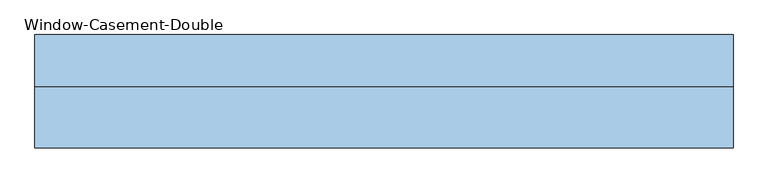
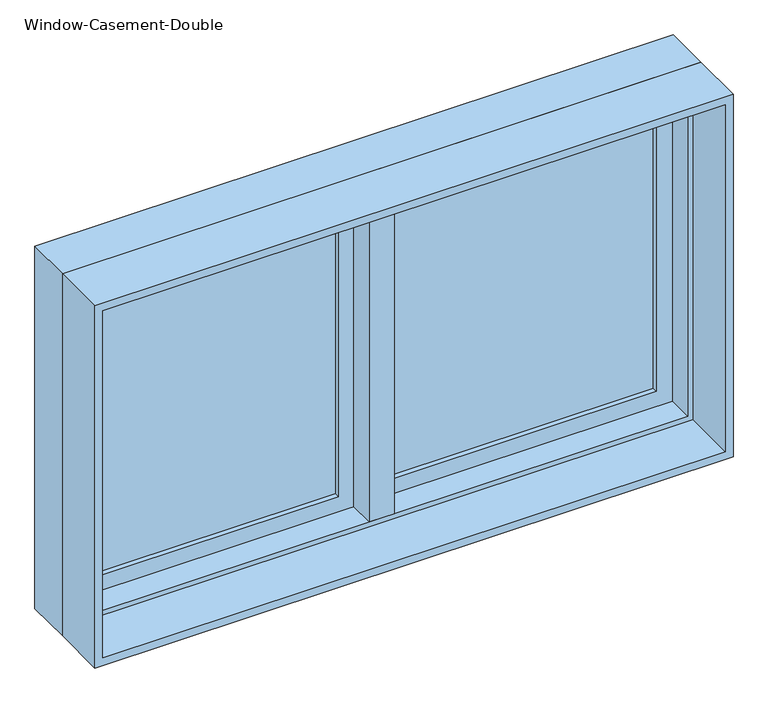
"""IFC4 building model written with IfcOpenShell, lengths in millimetres: window geometry, Window-Casement-Double."""

from ifc_helpers import new_model, si_unit, frame, origin, place, context, project, spatial, polyline, outline, extrude, faceted_brep, source, transform, mapped, element, save


def window_casement_double_c1d95f0f(model_context):
    return source(origin(), model_context, "Body", "SolidModel", [
        faceted_brep([(9.525, 133.35, 1816.1), (-9.525, 133.35, 1816.1), (-9.525, 82.55, 1816.1), (9.525, 82.55, 1816.1), (9.525, 133.35, 927.1), (9.525, 82.55, 927.1), (-9.525, 82.55, 927.1), (-9.525, 133.35, 927.1), (-9.525, 82.55, 946.15), (-9.525, 82.55, 1797.05), (-30.1625, 82.55, 946.15), (-30.1625, 82.55, 1797.05), (-30.1625, 19.05, 946.15), (-30.1625, 19.05, 1797.05), (30.1625, 19.05, 946.15), (30.1625, 19.05, 1797.05), (30.1625, 82.55, 946.15), (30.1625, 82.55, 1797.05), (9.525, 82.55, 946.15), (9.525, 82.55, 1797.05)], [[[0, 1, 2, 3]], [[4, 5, 6, 7]], [[1, 0, 4, 7]], [[2, 1, 7, 6, 8, 9]], [[9, 8, 10, 11]], [[11, 10, 12, 13]], [[13, 12, 14, 15]], [[15, 14, 16, 17]], [[17, 16, 18, 19]], [[0, 3, 19, 18, 5, 4]], [[18, 8, 6, 5]], [[9, 19, 3, 2]], [[8, 18, 16, 14, 12, 10]], [[19, 9, 11, 13, 15, 17]]]),
        extrude(outline(polyline([(-66.675, 114.3), (-66.675, 107.95), (-692.15, 107.95), (-692.15, 114.3), (-66.675, 114.3)])), frame((0.0, 0.0, 984.25), z_axis=(0.0, 0.0, 1.0), x_axis=(1.0, 0.0, 0.0)), (0.0, 0.0, 1.0), 774.7),
        extrude(outline(polyline([(-692.15, 95.25), (-692.15, 101.6), (-66.675, 101.6), (-66.675, 95.25), (-692.15, 95.25)])), frame((0.0, 0.0, 984.25), z_axis=(0.0, 0.0, 1.0), x_axis=(1.0, 0.0, 0.0)), (0.0, 0.0, 1.0), 774.7),
        extrude(outline(polyline([(692.15, 114.3), (692.15, 107.95), (66.675, 107.95), (66.675, 114.3), (692.15, 114.3)])), frame((0.0, 0.0, 984.25), z_axis=(0.0, 0.0, 1.0), x_axis=(1.0, 0.0, 0.0)), (0.0, 0.0, 1.0), 774.7),
        extrude(outline(polyline([(66.675, 95.25), (66.675, 101.6), (692.15, 101.6), (692.15, 95.25), (66.675, 95.25)])), frame((0.0, 0.0, 984.25), z_axis=(0.0, 0.0, 1.0), x_axis=(1.0, 0.0, 0.0)), (0.0, 0.0, 1.0), 774.7),
        extrude(outline(polyline([(1816.1, -749.3), (927.1, -749.3), (927.1, -9.525), (1816.1, -9.525), (1816.1, -749.3)]), holes=[polyline([(1758.95, -66.675), (984.25, -66.675), (984.25, -692.15), (1758.95, -692.15), (1758.95, -66.675)])]), frame((0.0, 82.55, 0.0), z_axis=(0.0, 1.0, 0.0), x_axis=(0.0, 0.0, 1.0)), (0.0, 0.0, 1.0), 44.45),
        extrude(outline(polyline([(927.1, 749.3), (1816.1, 749.3), (1816.1, 9.525), (927.1, 9.525), (927.1, 749.3)]), holes=[polyline([(984.25, 66.675), (1758.95, 66.675), (1758.95, 692.15), (984.25, 692.15), (984.25, 66.675)])]), frame((0.0, 82.55, 0.0), z_axis=(0.0, 1.0, 0.0), x_axis=(0.0, 0.0, 1.0)), (0.0, 0.0, 1.0), 44.45),
        extrude(outline(polyline([(1828.8, -762.0), (914.4, -762.0), (914.4, 762.0), (1828.8, 762.0), (1828.8, -762.0)]), holes=[polyline([(1809.75, 742.95), (933.45, 742.95), (933.45, -742.95), (1809.75, -742.95), (1809.75, 742.95)])]), frame((0.0, -114.3, 0.0), z_axis=(0.0, 1.0, 0.0), x_axis=(0.0, 0.0, 1.0)), (0.0, 0.0, 1.0), 133.35),
        faceted_brep([(730.25, 82.55, 1797.05), (730.25, 19.05, 1797.05), (-730.25, 19.05, 1797.05), (-730.25, 82.55, 1797.05), (749.3, 133.35, 1816.1), (749.3, 82.55, 1816.1), (-749.3, 82.55, 1816.1), (-749.3, 133.35, 1816.1), (762.0, 19.05, 1828.8), (762.0, 133.35, 1828.8), (-762.0, 133.35, 1828.8), (-762.0, 19.05, 1828.8), (-730.25, 19.05, 946.15), (-730.25, 82.55, 946.15), (-749.3, 82.55, 927.1), (-749.3, 133.35, 927.1), (-762.0, 133.35, 914.4), (-762.0, 19.05, 914.4), (730.25, 19.05, 946.15), (730.25, 82.55, 946.15), (749.3, 82.55, 927.1), (749.3, 133.35, 927.1), (762.0, 133.35, 914.4), (762.0, 19.05, 914.4)], [[[0, 1, 2, 3]], [[4, 5, 6, 7]], [[8, 9, 10, 11]], [[3, 2, 12, 13]], [[7, 6, 14, 15]], [[11, 10, 16, 17]], [[13, 12, 18, 19]], [[15, 14, 20, 21]], [[17, 16, 22, 23]], [[11, 17, 23, 8], [1, 18, 12, 2]], [[19, 18, 1, 0]], [[5, 20, 14, 6], [3, 13, 19, 0]], [[21, 20, 5, 4]], [[23, 22, 9, 8]], [[9, 22, 16, 10], [7, 15, 21, 4]]]),
    ])


if __name__ == "__main__":
    model = new_model("IFC4")
    model_context = context("Model", 3, world=origin())
    ifc_project = project(units=[si_unit("LENGTHUNIT", "METRE", prefix="MILLI")], contexts=[model_context])
    site = spatial("IfcSite", under=ifc_project)
    building = spatial("IfcBuilding", under=site)
    placement = place(None, origin())
    window_casement_double_shape = window_casement_double_c1d95f0f(model_context)
    element("IfcWindow", 1, ObjectType="Window-Casement-Double", at=placement, inside=building, context=model_context, shape_type="MappedRepresentation", body=[
        mapped(window_casement_double_shape, transform((0.0, 0.0, 0.0), x_axis=(1.0, 0.0, 0.0), y_axis=(0.0, 1.0, 0.0), z_axis=(0.0, 0.0, 1.0))),
    ])
    save(model, "model.ifc")

# Revit data of these elements
# Type "Window-Casement-Double"
#   Type Mark = "18"
#   Fire Rating = "0.5h"
#   Assembly Code = "B2020100"
#   Analytic Construction = "Double glazing - domestic"
#   Frame Extension [instance default] = 0' - 0 1/4"
#   Window Inset [instance default] = 0' - 0"
#   Wall Thickness [instance default] = 0' - 6"
#   Interior Wall Closure [instance default] = 0' - 2 1/4"
#   Half Width = 2' - 6"
#   Visual Light Transmittance = 0.81
#   Thermal Resistance (R) = 1.8146 (h·ft²·°F)/BTU
#   Solar Heat Gain Coefficient = 0.76
#   Rough Width = 5' - 0 1/2"
#   Rough Height = 3' - 0 1/2"
#   Height = 3' - 0"
#   Heat Transfer Coefficient (U) = 0.5511 BTU/(h·ft²·°F)
#   Exterior Wall Closure [instance default] = 0' - 1 1/4"
#   Extension Jamb [instance default] = 0' - 2 1/4"
#   Default Sill Height = 3' - 0"
#   Width = 5' - 0"
#   Muntin Visibility = yes
#   Interior Trim Visibility [instance default] = yes
#   Exterior Trim Visibility [instance default] = yes
#   Extension Jamb Visibility [instance default] = yes
#   Interior Trim Material = Wood - Stained
#   Muntin Pattern = Muntin Pattern_2x2 : Muntin Pattern_2x2
#   Interior Trim = Trim-Window-Interior-Flat : Picture Frame
#   Interior Frame Material = Wood - Stained
#   Glass Panel Material = Glass
#   Exterior Trim Material = Clad - White
#   Exterior Trim = Trim-Window-Exterior-Flat : with Sill
#   Exterior Frame Material = Clad - White
#   Wall Closure = (empty or 0)
# Element 1 (IfcWindow, "Window-Casement-Double")
#   Wall Thickness = 0' - 9"
#   Extension Jamb = 0' - 5 1/4"
#   Materials on its faces: "Wood - Stained", "Glass", "Clad - White"
# Materials
#   "Wood - Stained": class "Wood", colour RGB 224 178 126, transparency 0, Cost = 0
#   "Glass": class "Glass", colour RGB 0 128 192, transparency 0.75, Description = "Soda Lime Glass", Cost = 0
#   "Clad - White": class "Wood", colour RGB 242 242 238, transparency 0, Cost = 0
